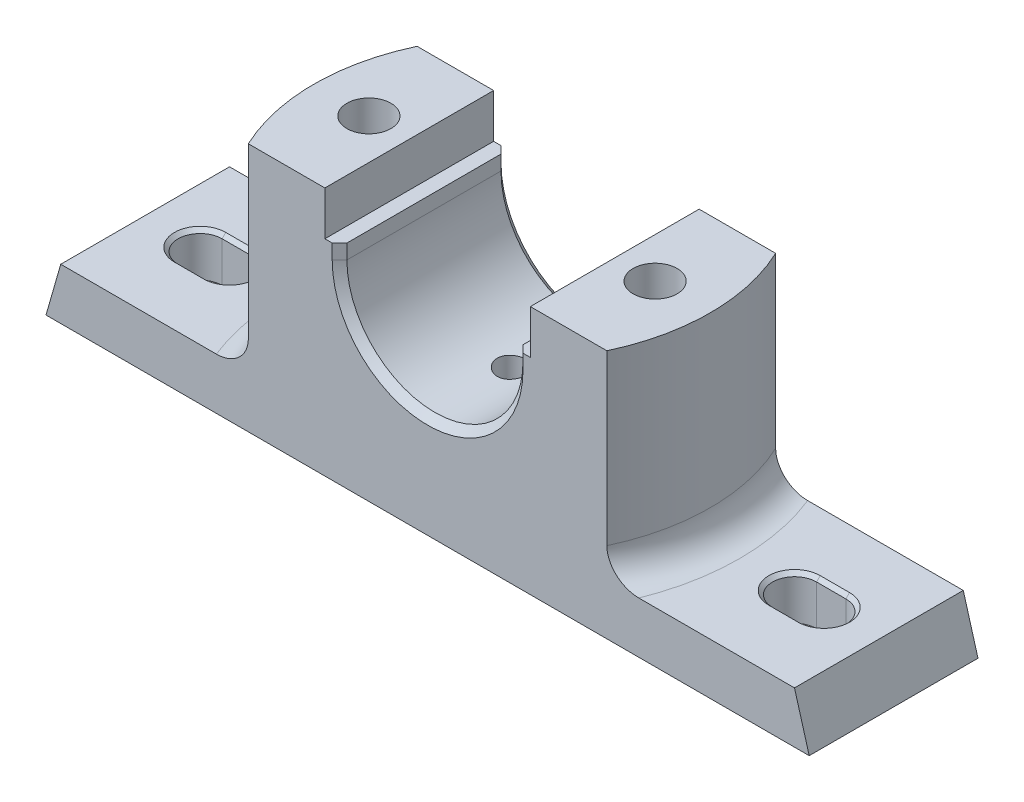
from build123d import *

# Parameters (mm, degrees)
BASE_PLATE_SKETCH_W             = 208
BASE_PLATE_SKETCH_H             = 46
BASE_PLATE_208X46X14_DEPTH      = 14
BASE_END_BEVEL_SKETCH_OUTSIDE_W = 252.698
BASE_END_BEVEL_SKETCH_OUTSIDE_H = 58.698
BASE_END_BEVELS_DEPTH           = 115.577484699
BEARING_PEDESTAL_DEPTH          = 46
UNDERSIDE_RELIEF_SKETCH_W       = 195
UNDERSIDE_RELIEF_SKETCH_H       = 36
UNDERSIDE_RELIEF_2MM_DEPTH      = 2
BEARING_BORE_SKETCH_W           = 28
BEARING_BORE_SKETCH_H           = 28
BEARING_BORE_CUT_DEPTH          = 10
MOUNTING_SLOTS_2X8_DEPTH        = 127.368508735
CAP_BOLT_HOLES_2X_12_D          = 12
PEDESTAL_CHAMFER_2MM_SIZE       = 2
SLOT_EDGE_CHAMFER_1MM_SIZE      = 1
DRILLED_HOLE_8_D                = 8
DRILLED_HOLE_8_DEPTH            = 36
PEDESTAL_PROFILE_CUT_DEPTH      = 54
PEDESTAL_BASE_FILLET_R8_R       = 8


with BuildPart() as part:
    # Base Plate Sketch → Base Plate 208x46x14 (new body)
    with BuildSketch(Plane(origin=(0, 0, 0), x_dir=(1, 0, 0), z_dir=(0, 1, 0))):
        Rectangle(BASE_PLATE_SKETCH_W, BASE_PLATE_SKETCH_H)
    extrude(amount=BASE_PLATE_208X46X14_DEPTH)

    # Base End Bevel Sketch outside → Base End Bevels (cut, through all)
    with BuildSketch(Plane.XY.offset(23)):
        with Locations((0, 7)):
            Rectangle(BASE_END_BEVEL_SKETCH_OUTSIDE_W, BASE_END_BEVEL_SKETCH_OUTSIDE_H)
        Polygon((-104, 0), (-99.985564599, 14), (99.985564599, 14), (104, 0), align=None, mode=Mode.SUBTRACT)
    extrude(amount=-BASE_END_BEVELS_DEPTH, mode=Mode.SUBTRACT)

    # Pedestal Sketch → Bearing Pedestal (add, through all)
    with BuildSketch(Plane.XY.offset(23)):
        with BuildLine():
            Line((-56, 14), (56, 14))
            Line((56, 14), (56, 68))
            Line((56, 68), (28, 68))
            Line((28, 68), (28, 56))
            Line((28, 56), (24, 56))
            Line((24, 56), (24, 52))
            ThreePointArc((24, 52), (0, 28), (-24, 52))
            Line((-24, 52), (-24, 56))
            Line((-24, 56), (-28, 56))
            Line((-28, 56), (-28, 68))
            Line((-28, 68), (-56, 68))
            Line((-56, 68), (-56, 14))
        make_face()
    extrude(amount=-BEARING_PEDESTAL_DEPTH)

    # Underside Relief Sketch → Underside Relief 2mm (cut)
    with BuildSketch(Plane.XZ):
        Rectangle(UNDERSIDE_RELIEF_SKETCH_W, UNDERSIDE_RELIEF_SKETCH_H)
    extrude(amount=-UNDERSIDE_RELIEF_2MM_DEPTH, mode=Mode.SUBTRACT)

    # Bearing Bore Sketch → Bearing Bore Cut (cut)
    with BuildSketch(Plane.XZ.offset(-2)):
        with Locations((39, 0)):
            Rectangle(BEARING_BORE_SKETCH_W, BEARING_BORE_SKETCH_H)
        with Locations((-39, 0)):
            Rectangle(BEARING_BORE_SKETCH_W, BEARING_BORE_SKETCH_H)
    extrude(amount=-BEARING_BORE_CUT_DEPTH, mode=Mode.SUBTRACT)

    # Mounting Slots Sketch → Mounting Slots 2x8 (cut, through all)
    with BuildSketch(Plane(origin=(0, 0, 0), x_dir=(1, 0, 0), z_dir=(0, 1, 0))):
        with BuildLine():
            Line((77, 6), (85, 6))
            ThreePointArc((85, 6), (91, 0), (85, -6))
            Line((85, -6), (77, -6))
            ThreePointArc((77, -6), (71, 0), (77, 6))
        make_face()
        with BuildLine():
            Line((-77, 6), (-85, 6))
            ThreePointArc((-85, 6), (-91, 0), (-85, -6))
            Line((-85, -6), (-77, -6))
            ThreePointArc((-77, -6), (-71, 0), (-77, 6))
        make_face()
    extrude(amount=MOUNTING_SLOTS_2X8_DEPTH, mode=Mode.SUBTRACT)

    # Cap Bolt Holes 2xØ12 (through all)
    with Locations(Plane(origin=(0, 12, 0), x_dir=(-1, 0, 0), z_dir=(0, -1, 0))):
        with Locations((-39, 0), (39, 0)):
            Hole(CAP_BOLT_HOLES_2X_12_D / 2)

    # Pedestal Chamfer 2mm
    pedestal_chamfer_2mm_edges = [part.edges().sort_by_distance(p)[0] for p in [
        (-24, 54, -23),
        (0, 28, -23),
        (24, 54, -23),
        (24, 54, 23),
        (0, 28, 23),
        (-24, 54, 23),
    ]]
    chamfer(pedestal_chamfer_2mm_edges, length=PEDESTAL_CHAMFER_2MM_SIZE)

    # Slot Edge Chamfer 1mm
    slot_edge_chamfer_1mm_edges = [part.edges().sort_by_distance(p)[0] for p in [
        (71, 14, 0),
        (81, 14, 6),
        (91, 14, 0),
        (81, 14, -6),
        (-71, 14, 0),
        (-81, 14, -6),
        (-91, 14, 0),
        (-81, 14, 6),
    ]]
    chamfer(slot_edge_chamfer_1mm_edges, length=SLOT_EDGE_CHAMFER_1MM_SIZE)

    # Drilled Hole Ø8
    with Locations(Plane(origin=(0, 56, 0), x_dir=(1, 0, 0), z_dir=(0, 1, 0))):
        with Locations((0, 0)):
            Hole(DRILLED_HOLE_8_D / 2, depth=DRILLED_HOLE_8_DEPTH)

    # Pedestal Profile Sketch → Pedestal Profile Cut (cut)
    with BuildSketch(Plane(origin=(0, 68, 0), x_dir=(1, 0, 0), z_dir=(0, 1, 0))):
        with BuildLine():
            Line((-56, -23), (-48.856934001, -23))
            ThreePointArc((-48.856934001, -23), (-54, 0), (-48.856934001, 23))
            Line((-48.856934001, 23), (-56, 23))
            Line((-56, 23), (-56, -23))
        make_face()
        with BuildLine():
            Line((48.856934001, -23), (56, -23))
            Line((56, -23), (56, 23))
            Line((56, 23), (48.856934001, 23))
            ThreePointArc((48.856934001, 23), (54, 0), (48.856934001, -23))
        make_face()
    extrude(amount=-PEDESTAL_PROFILE_CUT_DEPTH, mode=Mode.SUBTRACT)

    # Pedestal Base Fillet R8
    pedestal_base_fillet_r8_edges = [part.edges().sort_by_distance(p)[0] for p in [
        (-54, 14, 0),
        (54, 14, 0),
    ]]
    fillet(pedestal_base_fillet_r8_edges, radius=PEDESTAL_BASE_FILLET_R8_R)


solid = part.part
